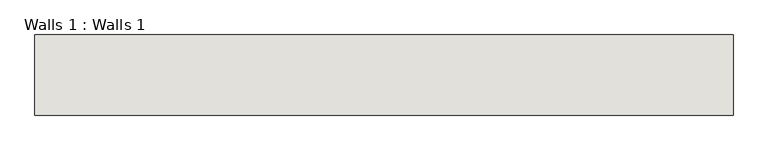
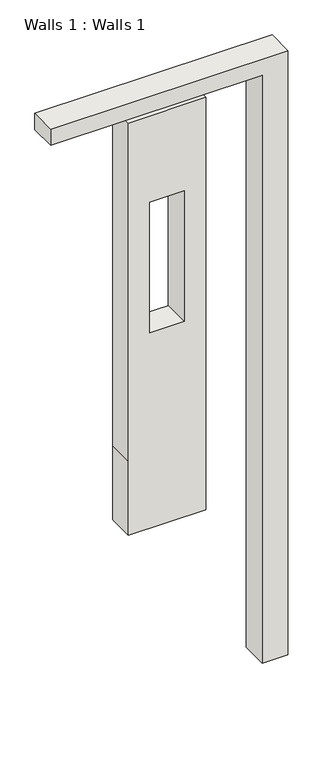
"""IFC4 building model written with IfcOpenShell, lengths in millimetres: wall geometry, Walls 1 : Walls 1."""

from ifc_helpers import new_model, si_unit, frame, origin, place, context, project, spatial, polyline, outline, extrude, source, transform, mapped, element, save


def walls_1_walls_1_cb3e8ea8(model_context):
    return source(origin(), model_context, "Body", "SweptSolid", [
        extrude(outline(polyline([(11277.6, -2789.0236868), (11277.6, -6980.0236868), (10972.8, -6980.0236868), (10972.8, -3246.2236868), (0.0, -3246.2236868), (0.0, -2789.0236868), (11277.6, -2789.0236868)])), frame((0.0, 5410.7832269, 0.0), z_axis=(0.0, 1.0, 0.0), x_axis=(0.0, 0.0, 1.0)), (0.0, 0.0, 1.0), 482.4338623),
        extrude(outline(polyline([(4585.3555883, -5608.4236868), (3213.7555883, -5608.4236868), (3213.7555883, -4236.8236868), (10909.9555883, -4236.8236868), (10909.9555883, -5608.4236868), (4585.3555883, -5608.4236868)]), holes=[polyline([(6866.3811024, -5232.7322745), (9304.7811024, -5232.7322745), (9304.7811024, -4623.1322745), (6866.3811024, -4623.1322745), (6866.3811024, -5232.7322745)])]), frame((0.0, 5410.7832269, 0.0), z_axis=(0.0, 1.0, 0.0), x_axis=(0.0, 0.0, 1.0)), (0.0, 0.0, 1.0), 482.4338623),
    ])


if __name__ == "__main__":
    model = new_model("IFC4")
    model_context = context("Model", 3, world=origin())
    ifc_project = project(units=[si_unit("LENGTHUNIT", "METRE", prefix="MILLI")], contexts=[model_context])
    site = spatial("IfcSite", under=ifc_project)
    building = spatial("IfcBuilding", under=site)
    placement = place(None, origin())
    walls_1_walls_1_shape = walls_1_walls_1_cb3e8ea8(model_context)
    element("IfcWall", 1, ObjectType="Walls 1 : Walls 1", at=placement, inside=building, context=model_context, shape_type="MappedRepresentation", body=[
        mapped(walls_1_walls_1_shape, transform((0.0, 0.0, 0.0), x_axis=(1.0, 0.0, 0.0), y_axis=(0.0, 1.0, 0.0), z_axis=(0.0, 0.0, 1.0))),
    ])
    save(model, "model.ifc")

# Revit data of these elements
# Element 1 (IfcWall, "Walls 1 : Walls 1")
#   Materials on its faces: "Default Wall"
# Materials
#   "Default Wall": colour RGB 128 128 128, transparency 0
